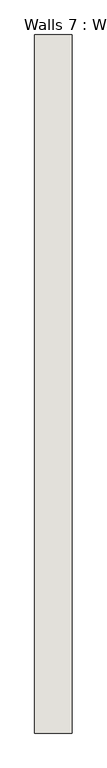
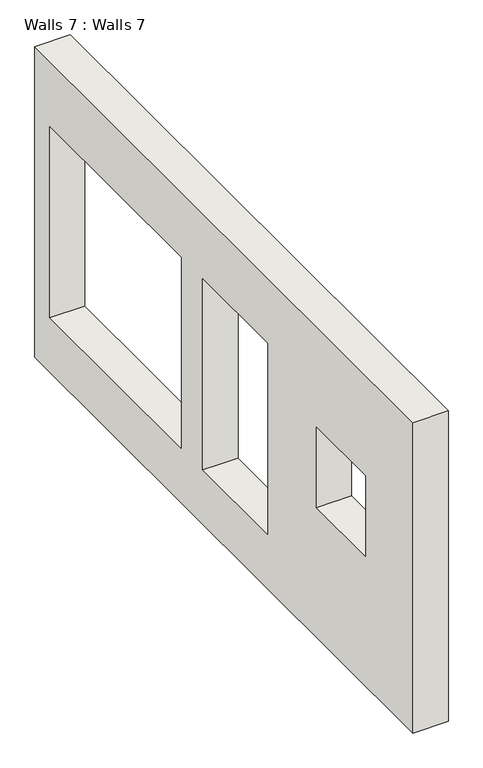
"""IFC4 building model written with IfcOpenShell, lengths in millimetres: wall geometry, Walls 7 : Walls 7."""

from ifc_helpers import new_model, si_unit, frame, origin, place, context, project, spatial, polyline, outline, extrude, source, transform, mapped, element, save


def walls_7_walls_7_b227ebcc(model_context):
    return source(origin(), model_context, "Body", "SweptSolid", [
        extrude(outline(polyline([(11358.0609482, 7315.2), (11358.0609482, 2608.8837371), (1960.0609482, 2608.8837371), (1960.0609482, 7315.2), (11358.0609482, 7315.2)]), holes=[polyline([(5580.0518123, 6324.9019988), (5580.0518123, 3429.3019988), (7185.0917513, 3429.3019988), (7185.0917513, 6324.9019988), (5580.0518123, 6324.9019988)]), polyline([(10990.2518123, 3429.3019988), (10990.2518123, 6324.9019988), (7724.717248, 6324.9019988), (7724.717248, 3429.3019988), (10990.2518123, 3429.3019988)]), polyline([(3140.4788247, 5791.2), (3140.4788247, 4572.0), (4359.6788247, 4572.0), (4359.6788247, 5791.2), (3140.4788247, 5791.2)])]), frame((1433.7254876, 0.0, 0.0), z_axis=(1.0, 0.0, 0.0), x_axis=(0.0, 1.0, 0.0)), (0.0, 0.0, 1.0), 504.5951336),
    ])


if __name__ == "__main__":
    model = new_model("IFC4")
    model_context = context("Model", 3, world=origin())
    ifc_project = project(units=[si_unit("LENGTHUNIT", "METRE", prefix="MILLI")], contexts=[model_context])
    site = spatial("IfcSite", under=ifc_project)
    building = spatial("IfcBuilding", under=site)
    placement = place(None, origin())
    walls_7_walls_7_shape = walls_7_walls_7_b227ebcc(model_context)
    element("IfcWall", 1, ObjectType="Walls 7 : Walls 7", at=placement, inside=building, context=model_context, shape_type="MappedRepresentation", body=[
        mapped(walls_7_walls_7_shape, transform((0.0, 0.0, 0.0), x_axis=(1.0, 0.0, 0.0), y_axis=(0.0, 1.0, 0.0), z_axis=(0.0, 0.0, 1.0))),
    ])
    save(model, "model.ifc")

# Revit data of these elements
# Element 1 (IfcWall, "Walls 7 : Walls 7")
#   Materials on its faces: "Default Wall"
# Materials
#   "Default Wall": colour RGB 128 128 128, transparency 0
